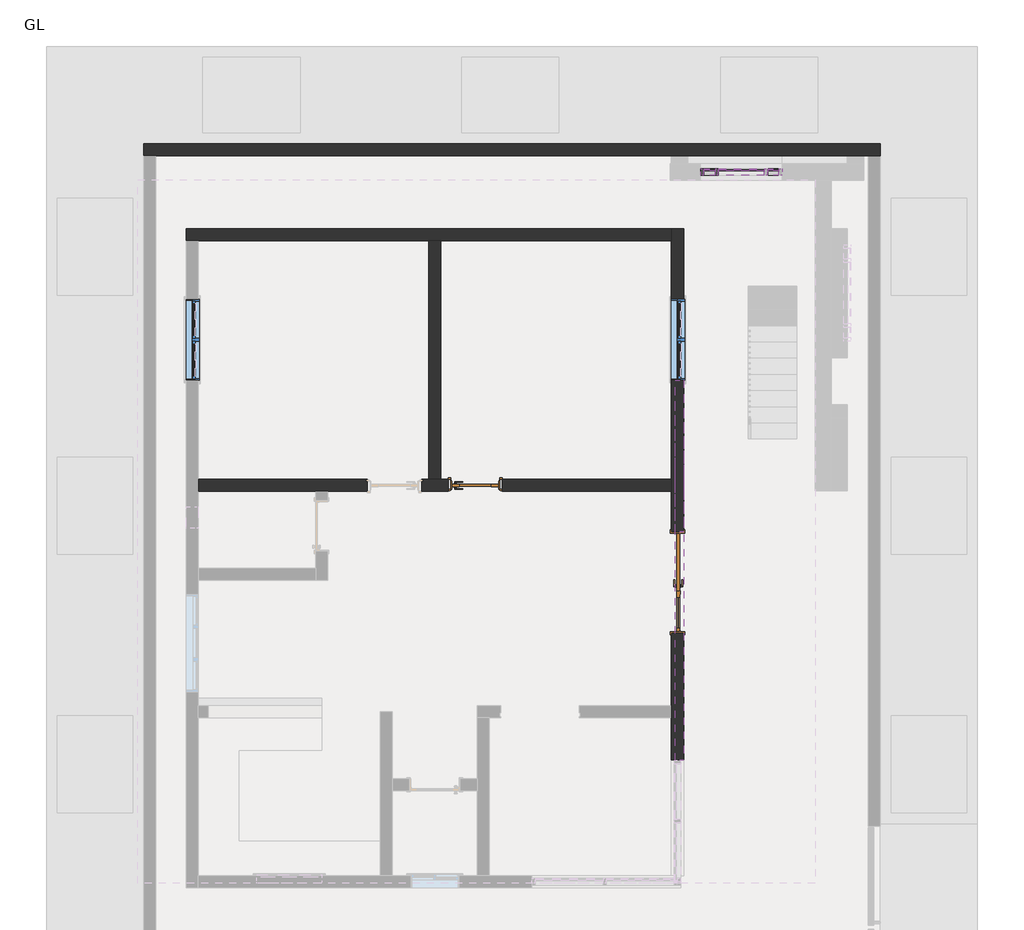
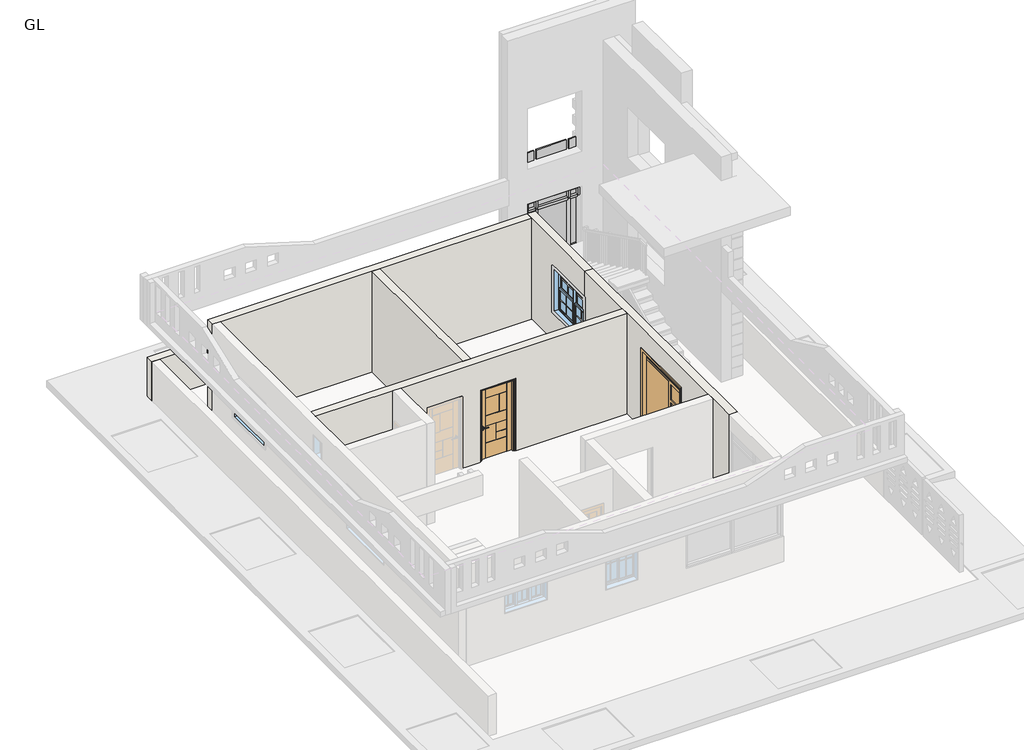
# One storey, part 2 of 4: 14 members, 10 proxies, 6 plates, 6 walls, 2 doors, 2 windows.
"""IFC4 building model written with IfcOpenShell, lengths in millimetres."""

from ifc_helpers import new_model, si_unit, frame, origin, origin_with_axes, place, context, project, spatial, polyline, outline, extrude, faceted_brep, transform, mapped, element, save
from components import main_entrance_door_11153_main_entrance_door_11153_94c2f9e1, single_modern_wooden_door_17379_single_modern_wooden_door_9761f21e, member_420b45ef, member_044eafc8, member_4491d118, member_a5966c2a, member_b00ab025, member_5d039c20, member_96c05505, member_82905deb, system_panel_glazed_a4d46631, system_panel_glazed_026653f5, system_panel_glazed_c2730be0, system_panel_glazed_e33957fc, system_panel_glazed_a01a9dc6, window_bf3e2632

model = new_model("IFC4")

# Units and contexts
model_context = context("Model", 3, world=origin())
ifc_project = project(units=[si_unit("LENGTHUNIT", "METRE", prefix="MILLI")], contexts=[model_context])

# Site, building, storey
site = spatial("IfcSite", under=ifc_project)
building = spatial("IfcBuilding", under=site)
storey = spatial("IfcBuildingStorey", under=building, Name="GL", Elevation=0.0)

# Proxies
placement = place(None, origin())
element("IfcBuildingElementProxy", 1, Name="Reveal", ObjectType="Reveal", at=placement, inside=storey, context=model_context, shape_type="SweptSolid", body=[
    extrude(outline(polyline([(-2365.7277598, 8208.9342801), (-2213.3277598, 8208.9342801), (-2213.3277598, 1052.4842801), (-2365.7277598, 1052.4842801), (-2365.7277598, 8208.9342801)])), frame((0.0, 0.0, 2819.4), z_axis=(0.0, 0.0, 1.0), x_axis=(1.0, 0.0, 0.0)), (0.0, 0.0, 1.0), 152.4),
])
element("IfcBuildingElementProxy", 2, Name="Reveal", ObjectType="Reveal", at=placement, inside=storey, context=model_context, shape_type="SweptSolid", body=[
    extrude(outline(polyline([(-2365.7277598, 8208.9342801), (-2213.3277598, 8208.9342801), (-2213.3277598, 5348.9342801), (-2365.7277598, 5348.9342801), (-2365.7277598, 8208.9342801)])), frame((0.0, 0.0, 152.4), z_axis=(0.0, 0.0, 1.0), x_axis=(1.0, 0.0, 0.0)), (0.0, 0.0, 1.0), 152.4),
    extrude(outline(polyline([(-2365.7277598, 3448.9342801), (-2213.3277598, 3448.9342801), (-2213.3277598, 1052.4842801), (-2365.7277598, 1052.4842801), (-2365.7277598, 3448.9342801)])), frame((0.0, 0.0, 152.4), z_axis=(0.0, 0.0, 1.0), x_axis=(1.0, 0.0, 0.0)), (0.0, 0.0, 1.0), 152.4),
])
element("IfcBuildingElementProxy", 3, Name="Reveal", ObjectType="Reveal", at=placement, inside=storey, context=model_context, shape_type="SweptSolid", body=[
    extrude(outline(polyline([(-2365.7277598, 8208.9342801), (-2213.3277598, 8208.9342801), (-2213.3277598, 1052.4842801), (-2365.7277598, 1052.4842801), (-2365.7277598, 8208.9342801)])), frame((0.0, 0.0, 2523.0666667), z_axis=(0.0, 0.0, 1.0), x_axis=(1.0, 0.0, 0.0)), (0.0, 0.0, 1.0), 152.4),
])
element("IfcBuildingElementProxy", 4, Name="Reveal", ObjectType="Reveal", at=placement, inside=storey, context=model_context, shape_type="SweptSolid", body=[
    extrude(outline(polyline([(-2365.7277598, 8208.9342801), (-2213.3277598, 8208.9342801), (-2213.3277598, 5348.9342801), (-2365.7277598, 5348.9342801), (-2365.7277598, 8208.9342801)])), frame((0.0, 0.0, 2226.7333333), z_axis=(0.0, 0.0, 1.0), x_axis=(1.0, 0.0, 0.0)), (0.0, 0.0, 1.0), 152.4),
    extrude(outline(polyline([(-2365.7277598, 3448.9342801), (-2213.3277598, 3448.9342801), (-2213.3277598, 1052.4842801), (-2365.7277598, 1052.4842801), (-2365.7277598, 3448.9342801)])), frame((0.0, 0.0, 2226.7333333), z_axis=(0.0, 0.0, 1.0), x_axis=(1.0, 0.0, 0.0)), (0.0, 0.0, 1.0), 152.4),
])
element("IfcBuildingElementProxy", 5, Name="Reveal", ObjectType="Reveal", at=placement, inside=storey, context=model_context, shape_type="SweptSolid", body=[
    extrude(outline(polyline([(-2365.7277598, 8208.9342801), (-2213.3277598, 8208.9342801), (-2213.3277598, 5348.9342801), (-2365.7277598, 5348.9342801), (-2365.7277598, 8208.9342801)])), frame((0.0, 0.0, 1930.4), z_axis=(0.0, 0.0, 1.0), x_axis=(1.0, 0.0, 0.0)), (0.0, 0.0, 1.0), 152.4),
    extrude(outline(polyline([(-2365.7277598, 3448.9342801), (-2213.3277598, 3448.9342801), (-2213.3277598, 1052.4842801), (-2365.7277598, 1052.4842801), (-2365.7277598, 3448.9342801)])), frame((0.0, 0.0, 1930.4), z_axis=(0.0, 0.0, 1.0), x_axis=(1.0, 0.0, 0.0)), (0.0, 0.0, 1.0), 152.4),
])
element("IfcBuildingElementProxy", 6, Name="Reveal", ObjectType="Reveal", at=placement, inside=storey, context=model_context, shape_type="SweptSolid", body=[
    extrude(outline(polyline([(-2365.7277598, 8208.9342801), (-2213.3277598, 8208.9342801), (-2213.3277598, 5348.9342801), (-2365.7277598, 5348.9342801), (-2365.7277598, 8208.9342801)])), frame((0.0, 0.0, 1634.0666667), z_axis=(0.0, 0.0, 1.0), x_axis=(1.0, 0.0, 0.0)), (0.0, 0.0, 1.0), 152.4),
    extrude(outline(polyline([(-2365.7277598, 3448.9342801), (-2213.3277598, 3448.9342801), (-2213.3277598, 1052.4842801), (-2365.7277598, 1052.4842801), (-2365.7277598, 3448.9342801)])), frame((0.0, 0.0, 1634.0666667), z_axis=(0.0, 0.0, 1.0), x_axis=(1.0, 0.0, 0.0)), (0.0, 0.0, 1.0), 152.4),
])
element("IfcBuildingElementProxy", 7, Name="Reveal", ObjectType="Reveal", at=placement, inside=storey, context=model_context, shape_type="SweptSolid", body=[
    extrude(outline(polyline([(-2365.7277598, 8208.9342801), (-2213.3277598, 8208.9342801), (-2213.3277598, 5348.9342801), (-2365.7277598, 5348.9342801), (-2365.7277598, 8208.9342801)])), frame((0.0, 0.0, 1337.7333333), z_axis=(0.0, 0.0, 1.0), x_axis=(1.0, 0.0, 0.0)), (0.0, 0.0, 1.0), 152.4),
    extrude(outline(polyline([(-2365.7277598, 3448.9342801), (-2213.3277598, 3448.9342801), (-2213.3277598, 1052.4842801), (-2365.7277598, 1052.4842801), (-2365.7277598, 3448.9342801)])), frame((0.0, 0.0, 1337.7333333), z_axis=(0.0, 0.0, 1.0), x_axis=(1.0, 0.0, 0.0)), (0.0, 0.0, 1.0), 152.4),
])
element("IfcBuildingElementProxy", 8, Name="Reveal", ObjectType="Reveal", at=placement, inside=storey, context=model_context, shape_type="SweptSolid", body=[
    extrude(outline(polyline([(-2365.7277598, 8208.9342801), (-2213.3277598, 8208.9342801), (-2213.3277598, 5348.9342801), (-2365.7277598, 5348.9342801), (-2365.7277598, 8208.9342801)])), frame((0.0, 0.0, 1041.4), z_axis=(0.0, 0.0, 1.0), x_axis=(1.0, 0.0, 0.0)), (0.0, 0.0, 1.0), 152.4),
    extrude(outline(polyline([(-2365.7277598, 3448.9342801), (-2213.3277598, 3448.9342801), (-2213.3277598, 1052.4842801), (-2365.7277598, 1052.4842801), (-2365.7277598, 3448.9342801)])), frame((0.0, 0.0, 1041.4), z_axis=(0.0, 0.0, 1.0), x_axis=(1.0, 0.0, 0.0)), (0.0, 0.0, 1.0), 152.4),
])
element("IfcBuildingElementProxy", 9, Name="Reveal", ObjectType="Reveal", at=placement, inside=storey, context=model_context, shape_type="SweptSolid", body=[
    extrude(outline(polyline([(-2365.7277598, 8208.9342801), (-2213.3277598, 8208.9342801), (-2213.3277598, 5348.9342801), (-2365.7277598, 5348.9342801), (-2365.7277598, 8208.9342801)])), frame((0.0, 0.0, 745.0666667), z_axis=(0.0, 0.0, 1.0), x_axis=(1.0, 0.0, 0.0)), (0.0, 0.0, 1.0), 152.4),
    extrude(outline(polyline([(-2365.7277598, 3448.9342801), (-2213.3277598, 3448.9342801), (-2213.3277598, 1052.4842801), (-2365.7277598, 1052.4842801), (-2365.7277598, 3448.9342801)])), frame((0.0, 0.0, 745.0666667), z_axis=(0.0, 0.0, 1.0), x_axis=(1.0, 0.0, 0.0)), (0.0, 0.0, 1.0), 152.4),
])
element("IfcBuildingElementProxy", 10, Name="Reveal", ObjectType="Reveal", at=placement, inside=storey, context=model_context, shape_type="SweptSolid", body=[
    extrude(outline(polyline([(-2365.7277598, 8208.9342801), (-2213.3277598, 8208.9342801), (-2213.3277598, 5348.9342801), (-2365.7277598, 5348.9342801), (-2365.7277598, 8208.9342801)])), frame((0.0, 0.0, 448.7333333), z_axis=(0.0, 0.0, 1.0), x_axis=(1.0, 0.0, 0.0)), (0.0, 0.0, 1.0), 152.4),
    extrude(outline(polyline([(-2365.7277598, 3448.9342801), (-2213.3277598, 3448.9342801), (-2213.3277598, 1052.4842801), (-2365.7277598, 1052.4842801), (-2365.7277598, 3448.9342801)])), frame((0.0, 0.0, 448.7333333), z_axis=(0.0, 0.0, 1.0), x_axis=(1.0, 0.0, 0.0)), (0.0, 0.0, 1.0), 152.4),
])

# Doors
main_entrance_door_11153_main_entrance_door_11153_shape = main_entrance_door_11153_main_entrance_door_11153_94c2f9e1(model_context)
element("IfcDoor", 11, ObjectType="Main_entrance_door_11153 : Main_entrance_door_11153", at=placement, inside=storey, context=model_context, shape_type="MappedRepresentation", body=[
    mapped(main_entrance_door_11153_main_entrance_door_11153_shape, transform((-2327.6277598, 4398.9342801, 0.0), x_axis=(0.0, -1.0, 0.0), y_axis=(1.0, 0.0, 0.0), z_axis=(0.0, 0.0, 1.0))),
])
single_modern_wooden_door_17379_single_modern_wooden_door_shape = single_modern_wooden_door_17379_single_modern_wooden_door_9761f21e(model_context)
element("IfcDoor", 12, ObjectType="Single_-_Modern_Wooden_Door_17379 : Single_-_Modern_Wooden_Door_17379", at=placement, inside=storey, context=model_context, shape_type="MappedRepresentation", body=[
    mapped(single_modern_wooden_door_17379_single_modern_wooden_door_shape, transform((-6137.6277598, 6227.7342801, 0.0), x_axis=(-1.0, 0.0, 0.0), y_axis=(0.0, -1.0, 0.0), z_axis=(0.0, 0.0, 1.0))),
])

# Members
member_shape = member_420b45ef(model_context)
element("IfcMember", 13, ObjectType="Rectangular Mullion : 2.5\" x 5\" rectangular", at=placement, inside=storey, context=model_context, shape_type="MappedRepresentation", body=[
    mapped(member_shape, transform((-1828.7123825, 12133.2342801, 2585.72), x_axis=(0.0, 0.0, 1.0), y_axis=(0.0, 1.0, 0.0), z_axis=(-1.0, 0.0, 0.0))),
])
element("IfcMember", 14, ObjectType="Rectangular Mullion : 2.5\" x 5\" rectangular", at=placement, inside=storey, context=model_context, shape_type="MappedRepresentation", body=[
    mapped(member_shape, transform((-627.5183629, 12133.2342801, 2585.72), x_axis=(0.0, 0.0, 1.0), y_axis=(0.0, 1.0, 0.0), z_axis=(-1.0, 0.0, 0.0))),
])
element("IfcMember", 15, ObjectType="Rectangular Mullion : 2.5\" x 5\" rectangular", at=placement, inside=storey, context=model_context, shape_type="MappedRepresentation", body=[
    mapped(member_shape, transform((-417.9683629, 12133.2342801, 767.08), x_axis=(0.0, 0.0, -1.0), y_axis=(0.0, 1.0, 0.0), z_axis=(1.0, 0.0, 0.0))),
])
element("IfcMember", 16, ObjectType="Rectangular Mullion : 2.5\" x 5\" rectangular", at=placement, inside=storey, context=model_context, shape_type="MappedRepresentation", body=[
    mapped(member_shape, transform((-1619.1623825, 12133.2342801, 767.08), x_axis=(0.0, 0.0, -1.0), y_axis=(0.0, 1.0, 0.0), z_axis=(1.0, 0.0, 0.0))),
])
member_2_shape = member_044eafc8(model_context)
element("IfcMember", 17, ObjectType="Rectangular Mullion : 2.5\" x 5\" rectangular", at=placement, inside=storey, context=model_context, shape_type="MappedRepresentation", body=[
    mapped(member_2_shape, transform((-354.4683629, 12133.2342801, 2585.72), x_axis=(1.0, 0.0, 0.0), y_axis=(0.0, 1.0, 0.0), z_axis=(0.0, 0.0, 1.0))),
])
member_3_shape = member_4491d118(model_context)
element("IfcMember", 18, ObjectType="Rectangular Mullion : 2.5\" x 5\" rectangular", at=placement, inside=storey, context=model_context, shape_type="MappedRepresentation", body=[
    mapped(member_3_shape, transform((-1892.2123825, 12133.2342801, 767.08), x_axis=(-1.0, 0.0, 0.0), y_axis=(0.0, 1.0, 0.0), z_axis=(0.0, 0.0, -1.0))),
])
member_4_shape = member_a5966c2a(model_context)
element("IfcMember", 19, ObjectType="Rectangular Mullion : 2.5\" x 5\" rectangular", at=placement, inside=storey, context=model_context, shape_type="MappedRepresentation", body=[
    mapped(member_4_shape, transform((-1828.7123825, 12133.2342801, 2291.08), x_axis=(0.0, 0.0, 1.0), y_axis=(0.0, 1.0, 0.0), z_axis=(-1.0, 0.0, 0.0))),
])
element("IfcMember", 20, ObjectType="Rectangular Mullion : 2.5\" x 5\" rectangular", at=placement, inside=storey, context=model_context, shape_type="MappedRepresentation", body=[
    mapped(member_4_shape, transform((-627.5183629, 12133.2342801, 2291.08), x_axis=(0.0, 0.0, 1.0), y_axis=(0.0, 1.0, 0.0), z_axis=(-1.0, 0.0, 0.0))),
])
member_5_shape = member_b00ab025(model_context)
element("IfcMember", 21, ObjectType="Rectangular Mullion : 2.5\" x 5\" rectangular", at=placement, inside=storey, context=model_context, shape_type="MappedRepresentation", body=[
    mapped(member_5_shape, transform((-1555.6623825, 12133.2342801, 2291.08), x_axis=(0.0, 0.0, 1.0), y_axis=(0.0, 1.0, 0.0), z_axis=(-1.0, 0.0, 0.0))),
])
member_6_shape = member_5d039c20(model_context)
element("IfcMember", 22, ObjectType="Rectangular Mullion : 2.5\" x 5\" rectangular", at=placement, inside=storey, context=model_context, shape_type="MappedRepresentation", body=[
    mapped(member_6_shape, transform((-659.2683629, 12133.2342801, 2585.72), x_axis=(1.0, 0.0, 0.0), y_axis=(0.0, 1.0, 0.0), z_axis=(0.0, 0.0, 1.0))),
])
element("IfcMember", 23, ObjectType="Rectangular Mullion : 2.5\" x 5\" rectangular", at=placement, inside=storey, context=model_context, shape_type="MappedRepresentation", body=[
    mapped(member_6_shape, transform((-1587.4123825, 12133.2342801, 2585.72), x_axis=(1.0, 0.0, 0.0), y_axis=(0.0, 1.0, 0.0), z_axis=(0.0, 0.0, 1.0))),
])
member_7_shape = member_96c05505(model_context)
element("IfcMember", 24, ObjectType="Rectangular Mullion : 2.5\" x 5\" rectangular", at=placement, inside=storey, context=model_context, shape_type="MappedRepresentation", body=[
    mapped(member_7_shape, transform((-1555.6623825, 12133.2342801, 2585.72), x_axis=(0.0, 0.0, 1.0), y_axis=(0.0, 1.0, 0.0), z_axis=(-1.0, 0.0, 0.0))),
])
element("IfcMember", 25, ObjectType="Rectangular Mullion : 2.5\" x 5\" rectangular", at=placement, inside=storey, context=model_context, shape_type="MappedRepresentation", body=[
    mapped(member_2_shape, transform((-1892.2123825, 12133.2342801, 2291.08), x_axis=(-1.0, 0.0, 0.0), y_axis=(0.0, 1.0, 0.0), z_axis=(0.0, 0.0, -1.0))),
])
member_8_shape = member_82905deb(model_context)
element("IfcMember", 26, ObjectType="Rectangular Mullion : 2.5\" x 5\" rectangular", at=placement, inside=storey, context=model_context, shape_type="MappedRepresentation", body=[
    mapped(member_8_shape, transform((-1587.4123825, 12133.2342801, 2291.08), x_axis=(1.0, 0.0, 0.0), y_axis=(0.0, 1.0, 0.0), z_axis=(0.0, 0.0, 1.0))),
])

# Plates
system_panel_glazed_shape = system_panel_glazed_a4d46631(model_context)
element("IfcPlate", 27, ObjectType="System Panel : Glazed", at=placement, inside=storey, context=model_context, shape_type="MappedRepresentation", body=[
    mapped(system_panel_glazed_shape, transform((-1723.9373825, 12133.2342801, 830.58), x_axis=(1.0, 0.0, 0.0), y_axis=(0.0, 1.0, 0.0), z_axis=(0.0, 0.0, 1.0))),
])
element("IfcPlate", 28, ObjectType="System Panel : Glazed", at=placement, inside=storey, context=model_context, shape_type="MappedRepresentation", body=[
    mapped(system_panel_glazed_shape, transform((-522.7433629, 12133.2342801, 830.58), x_axis=(1.0, 0.0, 0.0), y_axis=(0.0, 1.0, 0.0), z_axis=(0.0, 0.0, 1.0))),
])
system_panel_glazed_2_shape = system_panel_glazed_026653f5(model_context)
element("IfcPlate", 29, ObjectType="System Panel : Glazed", at=placement, inside=storey, context=model_context, shape_type="MappedRepresentation", body=[
    mapped(system_panel_glazed_2_shape, transform((-1723.9373825, 12133.2342801, 2322.83), x_axis=(1.0, 0.0, 0.0), y_axis=(0.0, 1.0, 0.0), z_axis=(0.0, 0.0, 1.0))),
])
system_panel_glazed_3_shape = system_panel_glazed_c2730be0(model_context)
element("IfcPlate", 30, ObjectType="System Panel : Glazed", at=placement, inside=storey, context=model_context, shape_type="MappedRepresentation", body=[
    mapped(system_panel_glazed_3_shape, transform((-522.7433629, 12133.2342801, 2322.83), x_axis=(1.0, 0.0, 0.0), y_axis=(0.0, 1.0, 0.0), z_axis=(0.0, 0.0, 1.0))),
])
system_panel_glazed_4_shape = system_panel_glazed_e33957fc(model_context)
element("IfcPlate", 31, ObjectType="System Panel : Glazed", at=placement, inside=storey, context=model_context, shape_type="MappedRepresentation", body=[
    mapped(system_panel_glazed_4_shape, transform((-1123.3403727, 12133.2342801, 830.58), x_axis=(1.0, 0.0, 0.0), y_axis=(0.0, 1.0, 0.0), z_axis=(0.0, 0.0, 1.0))),
])
system_panel_glazed_5_shape = system_panel_glazed_a01a9dc6(model_context)
element("IfcPlate", 32, ObjectType="System Panel : Glazed", at=placement, inside=storey, context=model_context, shape_type="MappedRepresentation", body=[
    mapped(system_panel_glazed_5_shape, transform((-1123.3403727, 12133.2342801, 2322.83), x_axis=(1.0, 0.0, 0.0), y_axis=(0.0, 1.0, 0.0), z_axis=(0.0, 0.0, 1.0))),
])

# Walls
element("IfcWall", 33, ObjectType="Generic - 9\"", at=placement, inside=storey, context=model_context, shape_type="Brep", body=[
    faceted_brep([(-11585.9277598, 10837.8342801, 0.0), (-11357.3277598, 10837.8342801, 0.0), (-7013.9277598, 10837.8342801, 0.0), (-6785.3277598, 10837.8342801, 0.0), (-2441.9277598, 10837.8342801, 0.0), (-2441.9277598, 10837.8342801, 3048.0), (-6785.3277598, 10837.8342801, 3048.0), (-7013.9277598, 10837.8342801, 3048.0), (-11357.3277598, 10837.8342801, 3048.0), (-11585.9277598, 10837.8342801, 3048.0), (-11585.9277598, 11066.4342801, 0.0), (-11585.9277598, 11066.4342801, 3048.0), (-2441.9277598, 11066.4342801, 3048.0), (-2441.9277598, 11066.4342801, 0.0)], [[[0, 1, 2, 3, 4, 5, 6, 7, 8, 9]], [[10, 11, 12, 13]], [[4, 3, 2, 1, 0, 10, 13]], [[9, 8, 7, 6, 5, 12, 11]], [[0, 9, 11, 10]], [[5, 4, 13, 12]]]),
])
element("IfcWall", 34, ObjectType="Generic - 9\"", at=placement, inside=storey, context=model_context, shape_type="Brep", body=[
    faceted_brep([(-2441.9277598, 11066.4342801, 0.0), (-2441.9277598, 10837.8342801, 0.0), (-2441.9277598, 8208.9342801, 0.0), (-2441.9277598, 8208.9342801, 914.4), (-2441.9277598, 9732.9342801, 914.4), (-2441.9277598, 9732.9342801, 2235.2), (-2441.9277598, 8208.9342801, 2235.2), (-2441.9277598, 8208.9342801, 3048.0), (-2441.9277598, 10837.8342801, 3048.0), (-2441.9277598, 11066.4342801, 3048.0), (-2213.3277598, 8208.9342801, 0.0), (-2213.3277598, 11066.4342801, 0.0), (-2213.3277598, 11066.4342801, 3048.0), (-2213.3277598, 8208.9342801, 3048.0), (-2213.3277598, 8208.9342801, 2971.8), (-2213.3277598, 8208.9342801, 2819.4), (-2213.3277598, 8208.9342801, 2675.4666667), (-2213.3277598, 8208.9342801, 2523.0666667), (-2213.3277598, 8208.9342801, 2379.1333333), (-2213.3277598, 8208.9342801, 2235.2), (-2213.3277598, 9732.9342801, 2235.2), (-2213.3277598, 9732.9342801, 914.4), (-2213.3277598, 8208.9342801, 914.4), (-2213.3277598, 8208.9342801, 897.4666667), (-2213.3277598, 8208.9342801, 745.0666667), (-2213.3277598, 8208.9342801, 601.1333333), (-2213.3277598, 8208.9342801, 448.7333333), (-2213.3277598, 8208.9342801, 304.8), (-2213.3277598, 8208.9342801, 152.4)], [[[0, 1, 2, 3, 4, 5, 6, 7, 8, 9]], [[10, 11, 12, 13, 14, 15, 16, 17, 18, 19, 20, 21, 22, 23, 24, 25, 26, 27, 28]], [[2, 1, 0, 11, 10]], [[2, 10, 28, 27, 26, 25, 24, 23, 22, 3]], [[13, 7, 6, 19, 18, 17, 16, 15, 14]], [[9, 8, 7, 13, 12]], [[0, 9, 12, 11]], [[20, 5, 4, 21]], [[21, 4, 3, 22]], [[5, 20, 19, 6]]]),
])
element("IfcWall", 35, ObjectType="Generic - 9\"", at=placement, inside=storey, context=model_context, shape_type="SweptSolid", body=[
    extrude(outline(polyline([(-7013.9277598, 6342.0342801), (-7013.9277598, 10837.8342801), (-6785.3277598, 10837.8342801), (-6785.3277598, 6342.0342801), (-7013.9277598, 6342.0342801)])), origin_with_axes(), (0.0, 0.0, 1.0), 3048.0),
])
element("IfcWall", 36, ObjectType="Generic - 9\"", at=placement, inside=storey, context=model_context, shape_type="Brep", body=[
    faceted_brep([(-2441.9277598, 6113.4342801, 3048.0), (-8918.9277598, 6113.4342801, 3048.0), (-9147.5277598, 6113.4342801, 3048.0), (-11357.3277598, 6113.4342801, 3048.0), (-11357.3277598, 6113.4342801, 0.0), (-9147.5277598, 6113.4342801, 0.0), (-8918.9277598, 6113.4342801, 0.0), (-8170.0246348, 6113.4342801, 0.0), (-8170.0246348, 6113.4342801, 2193.925), (-7150.4527598, 6113.4342801, 2193.925), (-7150.4527598, 6113.4342801, 0.0), (-6648.8027598, 6113.4342801, 0.0), (-6648.8027598, 6113.4342801, 2193.925), (-5629.2308848, 6113.4342801, 2193.925), (-5629.2308848, 6113.4342801, 0.0), (-2441.9277598, 6113.4342801, 0.0), (-11357.3277598, 6342.0342801, 3048.0), (-7013.9277598, 6342.0342801, 3048.0), (-6785.3277598, 6342.0342801, 3048.0), (-2441.9277598, 6342.0342801, 3048.0), (-2441.9277598, 6342.0342801, 0.0), (-5629.2308848, 6342.0342801, 0.0), (-5629.2308848, 6342.0342801, 2193.925), (-6648.8027598, 6342.0342801, 2193.925), (-6648.8027598, 6342.0342801, 0.0), (-6785.3277598, 6342.0342801, 0.0), (-7013.9277598, 6342.0342801, 0.0), (-7150.4527598, 6342.0342801, 0.0), (-7150.4527598, 6342.0342801, 2193.925), (-8170.0246348, 6342.0342801, 2193.925), (-8170.0246348, 6342.0342801, 0.0), (-11357.3277598, 6342.0342801, 0.0)], [[[0, 1, 2, 3, 4, 5, 6, 7, 8, 9, 10, 11, 12, 13, 14, 15]], [[16, 17, 18, 19, 20, 21, 22, 23, 24, 25, 26, 27, 28, 29, 30, 31]], [[20, 15, 14, 21]], [[4, 31, 30, 7, 6, 5]], [[10, 27, 26, 25, 24, 11]], [[3, 2, 1, 0, 19, 18, 17, 16]], [[0, 15, 20, 19]], [[4, 3, 16, 31]], [[9, 28, 27, 10]], [[28, 9, 8, 29]], [[29, 8, 7, 30]], [[23, 12, 11, 24]], [[12, 23, 22, 13]], [[13, 22, 21, 14]]]),
])
element("IfcWall", 37, ObjectType="Generic - 9\"", at=placement, inside=storey, context=model_context, shape_type="Brep", body=[
    faceted_brep([(-12386.0277598, 12438.0342801, 0.0), (-12157.4277598, 12438.0342801, 0.0), (1266.4722402, 12438.0342801, 0.0), (1495.0722402, 12438.0342801, 0.0), (1495.0722402, 12438.0342801, 1219.2), (1266.4722402, 12438.0342801, 1219.2), (-12157.4277598, 12438.0342801, 1219.2), (-12386.0277598, 12438.0342801, 1219.2), (-12386.0277598, 12666.6342801, 0.0), (-12386.0277598, 12666.6342801, 1219.2), (1495.0722402, 12666.6342801, 1219.2), (1495.0722402, 12666.6342801, 0.0)], [[[0, 1, 2, 3, 4, 5, 6, 7]], [[8, 9, 10, 11]], [[3, 2, 1, 0, 8, 11]], [[7, 6, 5, 4, 10, 9]], [[4, 3, 11, 10]], [[0, 7, 9, 8]]]),
])
element("IfcWall", 38, ObjectType="Generic - 9\"", at=placement, inside=storey, context=model_context, shape_type="Brep", body=[
    faceted_brep([(-2441.9277598, 8208.9342801, 3048.0), (-2441.9277598, 8208.9342801, 2235.2), (-2441.9277598, 8208.9342801, 914.4), (-2441.9277598, 8208.9342801, 0.0), (-2441.9277598, 6342.0342801, 0.0), (-2441.9277598, 6113.4342801, 0.0), (-2441.9277598, 5348.9342801, 0.0), (-2441.9277598, 5348.9342801, 2400.0), (-2441.9277598, 3448.9342801, 2400.0), (-2441.9277598, 3448.9342801, 0.0), (-2441.9277598, 2074.8342801, 0.0), (-2441.9277598, 1846.2342801, 0.0), (-2441.9277598, 1052.4842801, 0.0), (-2441.9277598, 1052.4842801, 3048.0), (-2441.9277598, 1846.2342801, 3048.0), (-2441.9277598, 2074.8342801, 3048.0), (-2441.9277598, 6113.4342801, 3048.0), (-2441.9277598, 6342.0342801, 3048.0), (-2213.3277598, 8208.9342801, 3048.0), (-2213.3277598, 1052.4842801, 3048.0), (-2213.3277598, 1052.4842801, 2971.8), (-2213.3277598, 8208.9342801, 2971.8), (-2213.3277598, 1052.4842801, 0.0), (-2213.3277598, 3448.9342801, 0.0), (-2213.3277598, 3448.9342801, 152.4), (-2213.3277598, 1052.4842801, 152.4), (-2213.3277598, 5348.9342801, 0.0), (-2213.3277598, 8208.9342801, 0.0), (-2213.3277598, 8208.9342801, 152.4), (-2213.3277598, 5348.9342801, 152.4), (-2213.3277598, 3448.9342801, 2400.0), (-2213.3277598, 5348.9342801, 2400.0), (-2213.3277598, 5348.9342801, 2379.1333333), (-2213.3277598, 8208.9342801, 2379.1333333), (-2213.3277598, 8208.9342801, 2523.0666667), (-2213.3277598, 1052.4842801, 2523.0666667), (-2213.3277598, 1052.4842801, 2379.1333333), (-2213.3277598, 3448.9342801, 2379.1333333), (-2213.3277598, 8208.9342801, 2819.4), (-2213.3277598, 1052.4842801, 2819.4), (-2213.3277598, 1052.4842801, 2675.4666667), (-2213.3277598, 8208.9342801, 2675.4666667), (-2213.3277598, 5348.9342801, 304.8), (-2213.3277598, 8208.9342801, 304.8), (-2213.3277598, 8208.9342801, 448.7333333), (-2213.3277598, 5348.9342801, 448.7333333), (-2213.3277598, 1052.4842801, 304.8), (-2213.3277598, 3448.9342801, 304.8), (-2213.3277598, 3448.9342801, 448.7333333), (-2213.3277598, 1052.4842801, 448.7333333), (-2213.3277598, 8208.9342801, 1930.4), (-2213.3277598, 5348.9342801, 1930.4), (-2213.3277598, 5348.9342801, 1786.4666667), (-2213.3277598, 8208.9342801, 1786.4666667), (-2213.3277598, 5348.9342801, 2082.8), (-2213.3277598, 8208.9342801, 2082.8), (-2213.3277598, 8208.9342801, 2226.7333333), (-2213.3277598, 5348.9342801, 2226.7333333), (-2213.3277598, 3448.9342801, 1930.4), (-2213.3277598, 1052.4842801, 1930.4), (-2213.3277598, 1052.4842801, 1786.4666667), (-2213.3277598, 3448.9342801, 1786.4666667), (-2213.3277598, 1052.4842801, 2082.8), (-2213.3277598, 3448.9342801, 2082.8), (-2213.3277598, 3448.9342801, 2226.7333333), (-2213.3277598, 1052.4842801, 2226.7333333), (-2213.3277598, 5348.9342801, 601.1333333), (-2213.3277598, 8208.9342801, 601.1333333), (-2213.3277598, 8208.9342801, 745.0666667), (-2213.3277598, 5348.9342801, 745.0666667), (-2213.3277598, 1052.4842801, 601.1333333), (-2213.3277598, 3448.9342801, 601.1333333), (-2213.3277598, 3448.9342801, 745.0666667), (-2213.3277598, 1052.4842801, 745.0666667), (-2213.3277598, 5348.9342801, 897.4666667), (-2213.3277598, 8208.9342801, 897.4666667), (-2213.3277598, 8208.9342801, 914.4), (-2213.3277598, 8208.9342801, 1041.4), (-2213.3277598, 5348.9342801, 1041.4), (-2213.3277598, 1052.4842801, 897.4666667), (-2213.3277598, 3448.9342801, 897.4666667), (-2213.3277598, 3448.9342801, 1041.4), (-2213.3277598, 1052.4842801, 1041.4), (-2213.3277598, 5348.9342801, 1193.8), (-2213.3277598, 8208.9342801, 1193.8), (-2213.3277598, 8208.9342801, 1337.7333333), (-2213.3277598, 5348.9342801, 1337.7333333), (-2213.3277598, 1052.4842801, 1193.8), (-2213.3277598, 3448.9342801, 1193.8), (-2213.3277598, 3448.9342801, 1337.7333333), (-2213.3277598, 1052.4842801, 1337.7333333), (-2213.3277598, 5348.9342801, 1490.1333333), (-2213.3277598, 8208.9342801, 1490.1333333), (-2213.3277598, 8208.9342801, 1634.0666667), (-2213.3277598, 5348.9342801, 1634.0666667), (-2213.3277598, 1052.4842801, 1490.1333333), (-2213.3277598, 3448.9342801, 1490.1333333), (-2213.3277598, 3448.9342801, 1634.0666667), (-2213.3277598, 1052.4842801, 1634.0666667), (-2365.7277598, 8208.9342801, 2971.8), (-2365.7277598, 8208.9342801, 2819.4), (-2365.7277598, 8208.9342801, 2675.4666667), (-2365.7277598, 8208.9342801, 2523.0666667), (-2365.7277598, 8208.9342801, 2379.1333333), (-2365.7277598, 8208.9342801, 2226.7333333), (-2365.7277598, 8208.9342801, 2082.8), (-2365.7277598, 8208.9342801, 1930.4), (-2365.7277598, 8208.9342801, 1786.4666667), (-2365.7277598, 8208.9342801, 1634.0666667), (-2365.7277598, 8208.9342801, 1490.1333333), (-2365.7277598, 8208.9342801, 1337.7333333), (-2365.7277598, 8208.9342801, 1193.8), (-2365.7277598, 8208.9342801, 1041.4), (-2365.7277598, 8208.9342801, 897.4666667), (-2365.7277598, 8208.9342801, 745.0666667), (-2365.7277598, 8208.9342801, 601.1333333), (-2365.7277598, 8208.9342801, 448.7333333), (-2365.7277598, 8208.9342801, 304.8), (-2365.7277598, 8208.9342801, 152.4), (-2365.7277598, 1052.4842801, 152.4), (-2365.7277598, 1052.4842801, 304.8), (-2365.7277598, 1052.4842801, 448.7333333), (-2365.7277598, 1052.4842801, 601.1333333), (-2365.7277598, 1052.4842801, 745.0666667), (-2365.7277598, 1052.4842801, 897.4666667), (-2365.7277598, 1052.4842801, 1041.4), (-2365.7277598, 1052.4842801, 1193.8), (-2365.7277598, 1052.4842801, 1337.7333333), (-2365.7277598, 1052.4842801, 1490.1333333), (-2365.7277598, 1052.4842801, 1634.0666667), (-2365.7277598, 1052.4842801, 1786.4666667), (-2365.7277598, 1052.4842801, 1930.4), (-2365.7277598, 1052.4842801, 2082.8), (-2365.7277598, 1052.4842801, 2226.7333333), (-2365.7277598, 1052.4842801, 2379.1333333), (-2365.7277598, 1052.4842801, 2523.0666667), (-2365.7277598, 1052.4842801, 2675.4666667), (-2365.7277598, 1052.4842801, 2819.4), (-2365.7277598, 1052.4842801, 2971.8), (-2365.7277598, 3448.9342801, 2379.1333333), (-2365.7277598, 3448.9342801, 2226.7333333), (-2365.7277598, 3448.9342801, 2082.8), (-2365.7277598, 3448.9342801, 1930.4), (-2365.7277598, 3448.9342801, 1786.4666667), (-2365.7277598, 3448.9342801, 1634.0666667), (-2365.7277598, 3448.9342801, 1490.1333333), (-2365.7277598, 3448.9342801, 1337.7333333), (-2365.7277598, 3448.9342801, 1193.8), (-2365.7277598, 3448.9342801, 1041.4), (-2365.7277598, 3448.9342801, 897.4666667), (-2365.7277598, 3448.9342801, 745.0666667), (-2365.7277598, 3448.9342801, 601.1333333), (-2365.7277598, 3448.9342801, 448.7333333), (-2365.7277598, 3448.9342801, 304.8), (-2365.7277598, 3448.9342801, 152.4), (-2365.7277598, 5348.9342801, 152.4), (-2365.7277598, 5348.9342801, 304.8), (-2365.7277598, 5348.9342801, 448.7333333), (-2365.7277598, 5348.9342801, 601.1333333), (-2365.7277598, 5348.9342801, 745.0666667), (-2365.7277598, 5348.9342801, 897.4666667), (-2365.7277598, 5348.9342801, 1041.4), (-2365.7277598, 5348.9342801, 1193.8), (-2365.7277598, 5348.9342801, 1337.7333333), (-2365.7277598, 5348.9342801, 1490.1333333), (-2365.7277598, 5348.9342801, 1634.0666667), (-2365.7277598, 5348.9342801, 1786.4666667), (-2365.7277598, 5348.9342801, 1930.4), (-2365.7277598, 5348.9342801, 2082.8), (-2365.7277598, 5348.9342801, 2226.7333333), (-2365.7277598, 5348.9342801, 2379.1333333)], [[[0, 1, 2, 3, 4, 5, 6, 7, 8, 9, 10, 11, 12, 13, 14, 15, 16, 17]], [[18, 19, 20, 21]], [[22, 23, 24, 25]], [[26, 27, 28, 29]], [[30, 31, 32, 33, 34, 35, 36, 37]], [[38, 39, 40, 41]], [[42, 43, 44, 45]], [[46, 47, 48, 49]], [[50, 51, 52, 53]], [[54, 55, 56, 57]], [[58, 59, 60, 61]], [[62, 63, 64, 65]], [[66, 67, 68, 69]], [[70, 71, 72, 73]], [[74, 75, 76, 77, 78]], [[79, 80, 81, 82]], [[83, 84, 85, 86]], [[87, 88, 89, 90]], [[91, 92, 93, 94]], [[95, 96, 97, 98]], [[3, 27, 26, 6, 5, 4]], [[22, 12, 11, 10, 9, 23]], [[3, 2, 1, 0, 18, 21, 99, 100, 38, 41, 101, 102, 34, 33, 103, 104, 56, 55, 105, 106, 50, 53, 107, 108, 93, 92, 109, 110, 85, 84, 111, 112, 77, 76, 75, 113, 114, 68, 67, 115, 116, 44, 43, 117, 118, 28, 27]], [[0, 17, 16, 15, 14, 13, 19, 18]], [[12, 22, 25, 119, 120, 46, 49, 121, 122, 70, 73, 123, 124, 79, 82, 125, 126, 87, 90, 127, 128, 95, 98, 129, 130, 60, 59, 131, 132, 62, 65, 133, 134, 36, 35, 135, 136, 40, 39, 137, 138, 20, 19, 13]], [[8, 30, 37, 139, 140, 64, 63, 141, 142, 58, 61, 143, 144, 97, 96, 145, 146, 89, 88, 147, 148, 81, 80, 149, 150, 72, 71, 151, 152, 48, 47, 153, 154, 24, 23, 9]], [[30, 8, 7, 31]], [[31, 7, 6, 26, 29, 155, 156, 42, 45, 157, 158, 66, 69, 159, 160, 74, 78, 161, 162, 83, 86, 163, 164, 91, 94, 165, 166, 52, 51, 167, 168, 54, 57, 169, 170, 32]], [[100, 137, 39, 38]], [[137, 100, 99, 138]], [[138, 99, 21, 20]], [[118, 155, 29, 28]], [[155, 118, 117, 156]], [[156, 117, 43, 42]], [[154, 119, 25, 24]], [[119, 154, 153, 120]], [[120, 153, 47, 46]], [[106, 167, 51, 50]], [[167, 106, 105, 168]], [[168, 105, 55, 54]], [[142, 131, 59, 58]], [[131, 142, 141, 132]], [[132, 141, 63, 62]], [[104, 169, 57, 56]], [[169, 104, 103, 170]], [[170, 103, 33, 32]], [[140, 133, 65, 64]], [[133, 140, 139, 134]], [[134, 139, 37, 36]], [[102, 135, 35, 34]], [[135, 102, 101, 136]], [[136, 101, 41, 40]], [[116, 157, 45, 44]], [[157, 116, 115, 158]], [[158, 115, 67, 66]], [[152, 121, 49, 48]], [[121, 152, 151, 122]], [[122, 151, 71, 70]], [[114, 159, 69, 68]], [[159, 114, 113, 160]], [[160, 113, 75, 74]], [[150, 123, 73, 72]], [[123, 150, 149, 124]], [[124, 149, 80, 79]], [[112, 161, 78, 77]], [[161, 112, 111, 162]], [[162, 111, 84, 83]], [[148, 125, 82, 81]], [[125, 148, 147, 126]], [[126, 147, 88, 87]], [[110, 163, 86, 85]], [[163, 110, 109, 164]], [[164, 109, 92, 91]], [[146, 127, 90, 89]], [[127, 146, 145, 128]], [[128, 145, 96, 95]], [[108, 165, 94, 93]], [[165, 108, 107, 166]], [[166, 107, 53, 52]], [[144, 129, 98, 97]], [[129, 144, 143, 130]], [[130, 143, 61, 60]]]),
])

# Windows
window_shape = window_bf3e2632(model_context)
element("IfcWindow", 39, ObjectType="Window-Single-Hung-Double : 60\" x 52\"", at=placement, inside=storey, context=model_context, shape_type="MappedRepresentation", body=[
    mapped(window_shape, transform((-11471.6277598, 8970.9342801, 0.0), x_axis=(0.0, -1.0, 0.0), y_axis=(1.0, 0.0, 0.0), z_axis=(0.0, 0.0, 1.0))),
])
element("IfcWindow", 40, ObjectType="Window-Single-Hung-Double : 60\" x 52\"", at=placement, inside=storey, context=model_context, shape_type="MappedRepresentation", body=[
    mapped(window_shape, transform((-2327.6277598, 8970.9342801, 0.0), x_axis=(0.0, -1.0, 0.0), y_axis=(1.0, 0.0, 0.0), z_axis=(0.0, 0.0, 1.0))),
])

save(model, "model.ifc")

# Revit data of these elements
# Type "Main_entrance_door_11153 : Main_entrance_door_11153"
#   Type Mark = "14"
#   Height = 7' - 10.48819"
#   Width = 6' - 2.80315"
#   Door Width = 3' - 7.30709"
#   Function = (empty or 0)
#   Wall Closure = (empty or 0)
# Type "Single_-_Modern_Wooden_Door_17379 : Single_-_Modern_Wooden_Door_17379"
#   Type Mark = "8"
#   Frame Projection Ext. = 0' - 1"
#   Frame Projection Int. = 0' - 1"
#   Frame Width = 0' - 2"
#   Height = 7' - 0"
#   Width = 3' - 0"
#   Handel = Stainless Steel AISI 304
#   Glass = Glass
#   Door Frame = Wood (Oak)
#   Door = Custom Walnut
#   Function = (empty or 0)
#   Wall Closure = (empty or 0)
# Type "Rectangular Mullion : 2.5\" x 5\" rectangular"
#   built-in parameter 1007304 = 0.416667 (stored number, unit not read)
#   built-in parameter 1007301 = 0.104167 (stored number, unit not read)
#   built-in parameter 1007300 = 0.104167 (stored number, unit not read)
# Type "System Panel : Glazed"
#   Construction Type Id = "GSP4R"
#   Analytic Construction = "1/8 in Pilkington single glazing"
#   Visual Light Transmittance = 0.9
#   Solar Heat Gain Coefficient = 0.86
#   Heat Transfer Coefficient (U) = 1.18115 BTU/(h·ft²·°F)
#   Define Thermal Properties by = 1
# Type "Generic - 9\""
#   Layers, outside or top first: 0' - 0 1/2" no material (function 4); 0' - 8" "Brick, Common" (function 1); 0' - 0 1/2" no material (function 5)
# Type "Window-Single-Hung-Double : 60\" x 52\""
#   Type Mark = "18"
#   Fire Rating = "0.5h"
#   Construction Type Id = "DG-DR"
#   Analytic Construction = "Double glazing - domestic"
#   Wall Thickness [instance default] = 0' - 6"
#   Window Inset [instance default] = 0' - 0"
#   Visual Light Transmittance = 0.81
#   Thermal Resistance (R) = 1.8146 (h·ft²·°F)/BTU
#   Solar Heat Gain Coefficient = 0.76
#   Muntin Width = 2' - 0 1/16"
#   Muntin Height = 1' - 10 1/8"
#   Interior Wall Closure [instance default] = 0' - 1 1/2"
#   Rough Width = 5' - 0 1/2"
#   Rough Height = 4' - 4 1/2"
#   Frame Extension [instance default] = 0' - 1 1/4"
#   Exterior Wall Closure [instance default] = 0' - 0 1/2"
#   Extension Jamb [instance default] = 0' - 1 1/2"
#   Heat Transfer Coefficient (U) = 0.5511 BTU/(h·ft²·°F)
#   Height = 4' - 4"
#   Width = 5' - 0"
#   Top Muntin Visibility = yes
#   Indicator Visibility [instance default] = yes
#   Extension Jamb Visibility [instance default] = yes
#   Interior Trim Visibility [instance default] = yes
#   Exterior Trim Visibility [instance default] = yes
#   Define Thermal Properties by = 1
#   Bottom Muntin Visibility = yes
#   Muntin Pattern = Muntin Pattern_2x2 : Muntin Pattern_2x2
#   Interior Trim = Trim-Window-Interior-Flat : Picture Frame
#   Interior Trim Material = Wood - Stained
#   Exterior Trim Material = Clad - White
#   Exterior Trim = Trim-Window-Exterior-Flat : with Sill
#   Glass Panel Material = Glass
#   Exterior Frame Material = Clad - White
#   Interior Frame Material = Wood - Stained
#   Wall Closure = (empty or 0)
# Element 11 (IfcDoor, "Main_entrance_door_11153 : Main_entrance_door_11153")
#   Phase Created = New Construction
#   Materials on its faces: "Glass", "Default"
# Element 12 (IfcDoor, "Single_-_Modern_Wooden_Door_17379 : Single_-_Modern_Wooden_Door_17379")
#   Phase Created = New Construction
#   Materials on its faces: "Stainless Steel AISI 304", "Custom Walnut", "Wood (Oak)", "Glass"
# Elements 13, 14, 15, 16, 17, 18, 19, 20, 21, 22, 23, 24, 25, 26 (IfcMember, "Rectangular Mullion : 2.5\" x 5\" rectangular")
#   Phase Created = New Construction
#   Materials on its faces: "Aluminum"
# Elements 27, 28, 29, 30, 31, 32 (IfcPlate, "System Panel : Glazed")
#   Phase Created = New Construction
#   Materials on its faces: "Glass"
# Elements 33, 34, 35, 36, 38 (IfcWall, "Generic - 9\"")
#   Top Offset = -0' - 6"
#   Base Offset = 0' - 0"
#   wall height = 10' - 0"
#   Phase Created = New Construction
#   Base Constraint = GL
#   Top Constraint = 1st floor
#   Materials on its faces: "Default Wall"
# Element 37 (IfcWall, "Generic - 9\"")
#   Top Offset = -0' - 6"
#   Base Offset = 0' - 0"
#   Unconnected Height = 4' - 0"
#   wall height = 4' - 0"
#   Phase Created = New Construction
#   Base Constraint = GL
#   Materials on its faces: "Default Wall"
# Element 39 (IfcWindow, "Window-Single-Hung-Double : 60\" x 52\"")
#   Mark = "2"
#   Window Inset = 0' - 0"
#   Interior Wall Closure = 0' - 1 1/2"
#   Frame Extension = 0' - 1 1/4"
#   Exterior Wall Closure = 0' - 0 1/2"
#   Interior Trim Visibility = yes
#   Indicator Visibility = yes
#   Exterior Trim Visibility = yes
#   Phase Created = New Construction
#   Materials on its faces: "Wood - Stained", "Glass", "Clad - White"
# Element 40 (IfcWindow, "Window-Single-Hung-Double : 60\" x 52\"")
#   Mark = "3"
#   Window Inset = 0' - 0"
#   Interior Wall Closure = 0' - 1 1/2"
#   Frame Extension = 0' - 1 1/4"
#   Exterior Wall Closure = 0' - 0 1/2"
#   Interior Trim Visibility = yes
#   Indicator Visibility = yes
#   Exterior Trim Visibility = yes
#   Phase Created = New Construction
#   Materials on its faces: "Wood - Stained", "Glass", "Clad - White"
# Materials
#   "Stainless Steel AISI 304": class "Metal", colour RGB 244 244 244, transparency 0, Description = "Stainless Steel 18/8", Cost = 0
#   "Glass": class "Glass", colour RGB 0 128 192, transparency 0.75, Description = "Soda Lime Glass", Cost = 0
#   "Wood (Oak)": class "Wood", colour RGB 132 88 61, transparency 0, Description = "Physical material.", Cost = 0
#   "Custom Walnut": class "Wood", colour RGB 95 44 25, transparency 0, Description = "Juglans Nigra", Cost = 0
#   "Brick, Common": class "Masonry", colour RGB 85 47 55, transparency 0, Description = "Common brick", Cost = 0
#   "Wood - Stained": class "Wood", colour RGB 224 178 126, transparency 0, Cost = 0
#   "Clad - White": class "Wood", colour RGB 242 242 238, transparency 0, Cost = 0
#   "Default": colour RGB 127 127 127, transparency 0, Cost = 0
#   "Aluminum": class "Metal", colour RGB 247 247 247, transparency 0, Description = "Aluminum 6061", Cost = 0
#   "Default Wall": colour RGB 128 128 128, transparency 0, Cost = 0
